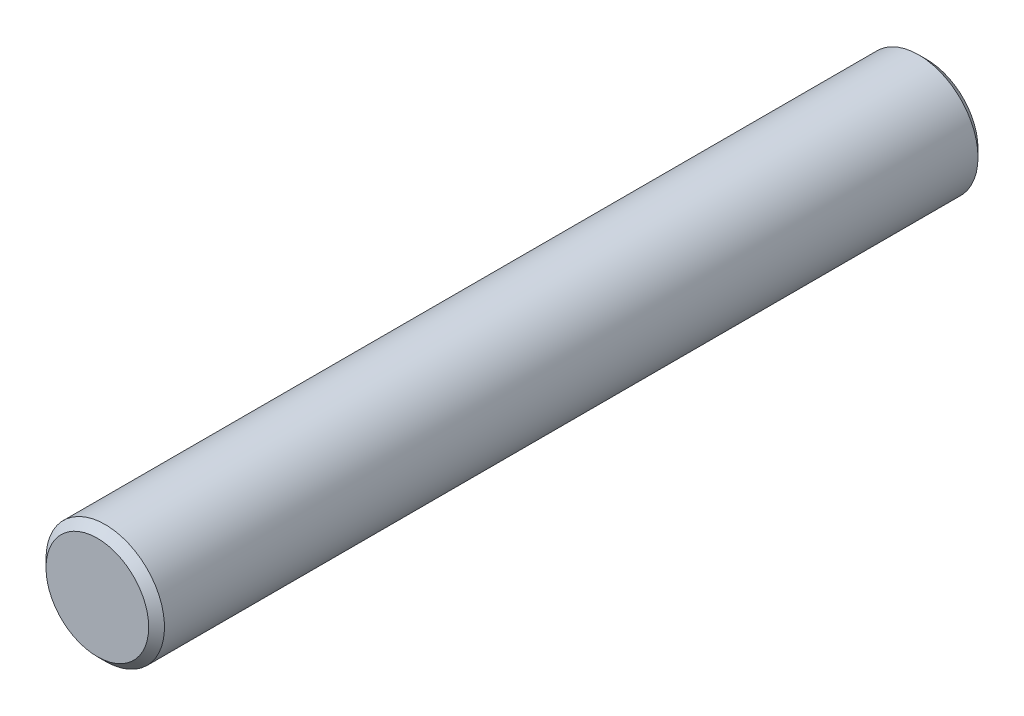
ISO-10303-21;
HEADER;
FILE_DESCRIPTION(('STEP AP214'),'2;1');
FILE_NAME('part.step','',(''),(''),'','','');
FILE_SCHEMA(('AUTOMOTIVE_DESIGN { 1 0 10303 214 1 1 1 1 }'));
ENDSEC;
DATA;
#1=APPLICATION_CONTEXT('core data for automotive mechanical design processes');
#2=APPLICATION_PROTOCOL_DEFINITION('international standard','automotive_design',2000,#1);
#3=PRODUCT_CONTEXT('',#1,'mechanical');
#4=PRODUCT('Part','Part','',(#3));
#5=PRODUCT_RELATED_PRODUCT_CATEGORY('part','',(#4));
#6=PRODUCT_DEFINITION_FORMATION('','',#4);
#7=PRODUCT_DEFINITION_CONTEXT('part definition',#1,'design');
#8=PRODUCT_DEFINITION('design','',#6,#7);
#9=PRODUCT_DEFINITION_SHAPE('','',#8);
#10=(LENGTH_UNIT() NAMED_UNIT(*) SI_UNIT(.MILLI.,.METRE.));
#11=(NAMED_UNIT(*) PLANE_ANGLE_UNIT() SI_UNIT($,.RADIAN.));
#12=(NAMED_UNIT(*) SI_UNIT($,.STERADIAN.) SOLID_ANGLE_UNIT());
#13=UNCERTAINTY_MEASURE_WITH_UNIT(LENGTH_MEASURE(1.E-05),#10,'distance_accuracy_value','');
#14=(GEOMETRIC_REPRESENTATION_CONTEXT(3) GLOBAL_UNCERTAINTY_ASSIGNED_CONTEXT((#13)) GLOBAL_UNIT_ASSIGNED_CONTEXT((#10,
#11,#12)) REPRESENTATION_CONTEXT('',''));
#15=CARTESIAN_POINT('',(0.,0.,0.));
#16=DIRECTION('',(0.,0.,1.));
#17=DIRECTION('',(1.,0.,0.));
#18=AXIS2_PLACEMENT_3D('',#15,#16,#17);
#19=CARTESIAN_POINT('',(0.,0.,10.5));
#20=DIRECTION('',(0.,0.,-1.));
#21=DIRECTION('',(-1.,0.,0.));
#22=AXIS2_PLACEMENT_3D('',#19,#20,#21);
#23=CYLINDRICAL_SURFACE('',#22,1.5);
#24=CARTESIAN_POINT('',(0.,0.,-10.3));
#25=DIRECTION('',(0.,0.,1.));
#26=DIRECTION('',(1.,0.,0.));
#27=AXIS2_PLACEMENT_3D('',#24,#25,#26);
#28=CIRCLE('',#27,1.5);
#29=CARTESIAN_POINT('',(-1.5,0.,-10.3));
#30=VERTEX_POINT('',#29);
#31=EDGE_CURVE('E51',#30,#30,#28,.T.);
#32=CARTESIAN_POINT('',(0.,0.,10.3));
#33=DIRECTION('',(0.,0.,1.));
#34=DIRECTION('',(1.,0.,0.));
#35=AXIS2_PLACEMENT_3D('',#32,#33,#34);
#36=CIRCLE('',#35,1.5);
#37=CARTESIAN_POINT('',(-1.5,0.,10.3));
#38=VERTEX_POINT('',#37);
#39=EDGE_CURVE('E54',#38,#38,#36,.F.);
#40=CARTESIAN_POINT('',(-1.5,0.,-10.3));
#41=CARTESIAN_POINT('',(-1.5,0.,-10.0854166666666));
#42=CARTESIAN_POINT('',(-1.5,0.,-9.87083333333331));
#43=CARTESIAN_POINT('',(-1.5,0.,-9.44166666666665));
#44=CARTESIAN_POINT('',(-1.5,0.,-9.22708333333332));
#45=CARTESIAN_POINT('',(-1.5,0.,-8.79791666666665));
#46=CARTESIAN_POINT('',(-1.5,0.,-8.58333333333331));
#47=CARTESIAN_POINT('',(-1.5,0.,-8.15416666666665));
#48=CARTESIAN_POINT('',(-1.5,0.,-7.93958333333331));
#49=CARTESIAN_POINT('',(-1.5,0.,-7.51041666666665));
#50=CARTESIAN_POINT('',(-1.5,0.,-7.29583333333331));
#51=CARTESIAN_POINT('',(-1.5,0.,-6.86666666666665));
#52=CARTESIAN_POINT('',(-1.5,0.,-6.65208333333332));
#53=CARTESIAN_POINT('',(-1.5,0.,-6.22291666666665));
#54=CARTESIAN_POINT('',(-1.5,0.,-6.00833333333332));
#55=CARTESIAN_POINT('',(-1.5,0.,-5.57916666666665));
#56=CARTESIAN_POINT('',(-1.5,0.,-5.36458333333332));
#57=CARTESIAN_POINT('',(-1.5,0.,-4.93541666666665));
#58=CARTESIAN_POINT('',(-1.5,0.,-4.72083333333332));
#59=CARTESIAN_POINT('',(-1.5,0.,-4.29166666666665));
#60=CARTESIAN_POINT('',(-1.5,0.,-4.07708333333332));
#61=CARTESIAN_POINT('',(-1.5,0.,-3.64791666666665));
#62=CARTESIAN_POINT('',(-1.5,0.,-3.43333333333332));
#63=CARTESIAN_POINT('',(-1.5,0.,-3.00416666666665));
#64=CARTESIAN_POINT('',(-1.5,0.,-2.78958333333332));
#65=CARTESIAN_POINT('',(-1.5,0.,-2.36041666666665));
#66=CARTESIAN_POINT('',(-1.5,0.,-2.14583333333332));
#67=CARTESIAN_POINT('',(-1.5,0.,-1.71666666666665));
#68=CARTESIAN_POINT('',(-1.5,0.,-1.50208333333332));
#69=CARTESIAN_POINT('',(-1.5,0.,-1.07291666666665));
#70=CARTESIAN_POINT('',(-1.5,0.,-0.85833333333332));
#71=CARTESIAN_POINT('',(-1.5,0.,-0.429166666666653));
#72=CARTESIAN_POINT('',(-1.5,0.,-0.21458333333332));
#73=CARTESIAN_POINT('',(-1.5,0.,0.214583333333347));
#74=CARTESIAN_POINT('',(-1.5,0.,0.429166666666681));
#75=CARTESIAN_POINT('',(-1.5,0.,0.858333333333347));
#76=CARTESIAN_POINT('',(-1.5,0.,1.07291666666668));
#77=CARTESIAN_POINT('',(-1.5,0.,1.50208333333335));
#78=CARTESIAN_POINT('',(-1.5,0.,1.71666666666668));
#79=CARTESIAN_POINT('',(-1.5,0.,2.14583333333335));
#80=CARTESIAN_POINT('',(-1.5,0.,2.36041666666668));
#81=CARTESIAN_POINT('',(-1.5,0.,2.78958333333335));
#82=CARTESIAN_POINT('',(-1.5,0.,3.00416666666668));
#83=CARTESIAN_POINT('',(-1.5,0.,3.43333333333335));
#84=CARTESIAN_POINT('',(-1.5,0.,3.64791666666668));
#85=CARTESIAN_POINT('',(-1.5,0.,4.07708333333334));
#86=CARTESIAN_POINT('',(-1.5,0.,4.29166666666668));
#87=CARTESIAN_POINT('',(-1.5,0.,4.72083333333334));
#88=CARTESIAN_POINT('',(-1.5,0.,4.93541666666668));
#89=CARTESIAN_POINT('',(-1.5,0.,5.36458333333334));
#90=CARTESIAN_POINT('',(-1.5,0.,5.57916666666668));
#91=CARTESIAN_POINT('',(-1.5,0.,6.00833333333334));
#92=CARTESIAN_POINT('',(-1.5,0.,6.22291666666668));
#93=CARTESIAN_POINT('',(-1.5,0.,6.65208333333334));
#94=CARTESIAN_POINT('',(-1.5,0.,6.86666666666668));
#95=CARTESIAN_POINT('',(-1.5,0.,7.29583333333334));
#96=CARTESIAN_POINT('',(-1.5,0.,7.51041666666667));
#97=CARTESIAN_POINT('',(-1.5,0.,7.93958333333334));
#98=CARTESIAN_POINT('',(-1.5,0.,8.15416666666668));
#99=CARTESIAN_POINT('',(-1.5,0.,8.58333333333334));
#100=CARTESIAN_POINT('',(-1.5,0.,8.79791666666668));
#101=CARTESIAN_POINT('',(-1.5,0.,9.22708333333334));
#102=CARTESIAN_POINT('',(-1.5,0.,9.44166666666668));
#103=CARTESIAN_POINT('',(-1.5,0.,9.87083333333334));
#104=CARTESIAN_POINT('',(-1.5,0.,10.0854166666667));
#105=CARTESIAN_POINT('',(-1.5,0.,10.3));
#106=B_SPLINE_CURVE_WITH_KNOTS('',3,(#40,#41,#42,#43,#44,#45,#46,#47,#48,#49,#50,#51,#52,#53,
#54,#55,#56,#57,#58,#59,#60,#61,#62,#63,#64,#65,#66,#67,#68,#69,#70,#71,#72,#73,#74,#75,#76,#77,
#78,#79,#80,#81,#82,#83,#84,#85,#86,#87,#88,#89,#90,#91,#92,#93,#94,#95,#96,#97,#98,#99,#100,
#101,#102,#103,#104,#105),.UNSPECIFIED.,.F.,.F.,(4,2,2,2,2,2,2,2,2,2,2,2,2,2,2,2,2,2,2,2,2,2,2,
2,2,2,2,2,2,2,2,2,4),(0.,0.643749999999998,1.2875,1.93125,2.575,3.21875,3.8625,4.50625,5.15,
5.79375,6.4375,7.08125,7.725,8.36875,9.01249999999999,9.65624999999999,10.3,10.94375,11.5875,
12.23125,12.875,13.51875,14.1625,14.80625,15.45,16.09375,16.7375,17.38125,18.025,18.66875,
19.3125,19.95625,20.6),.UNSPECIFIED.);
#107=EDGE_CURVE('BSEAM39',#30,#38,#106,.T.);
#108=ORIENTED_EDGE('',*,*,#31,.T.);
#109=ORIENTED_EDGE('',*,*,#39,.T.);
#110=ORIENTED_EDGE('',*,*,#107,.T.);
#111=ORIENTED_EDGE('',*,*,#107,.F.);
#112=EDGE_LOOP('',(#108,#110,#109,#111));
#113=FACE_BOUND('',#112,.T.);
#114=ADVANCED_FACE('F39',(#113),#23,.T.);
#115=CARTESIAN_POINT('',(0.,0.,10.5));
#116=DIRECTION('',(0.,0.,1.));
#117=DIRECTION('',(1.,0.,0.));
#118=AXIS2_PLACEMENT_3D('',#115,#116,#117);
#119=PLANE('',#118);
#120=CARTESIAN_POINT('',(0.,0.,10.5));
#121=DIRECTION('',(0.,0.,1.));
#122=DIRECTION('',(1.,0.,0.));
#123=AXIS2_PLACEMENT_3D('',#120,#121,#122);
#124=CIRCLE('',#123,1.30000000000001);
#125=CARTESIAN_POINT('',(1.30000000000001,0.,10.5));
#126=VERTEX_POINT('',#125);
#127=EDGE_CURVE('E10',#126,#126,#124,.T.);
#128=ORIENTED_EDGE('',*,*,#127,.T.);
#129=EDGE_LOOP('',(#128));
#130=FACE_BOUND('',#129,.T.);
#131=ADVANCED_FACE('F72',(#130),#119,.T.);
#132=CARTESIAN_POINT('',(0.,0.,-10.5));
#133=DIRECTION('',(0.,0.,1.));
#134=DIRECTION('',(1.,0.,0.));
#135=AXIS2_PLACEMENT_3D('',#132,#133,#134);
#136=PLANE('',#135);
#137=CARTESIAN_POINT('',(0.,0.,-10.5));
#138=DIRECTION('',(0.,0.,1.));
#139=DIRECTION('',(1.,0.,0.));
#140=AXIS2_PLACEMENT_3D('',#137,#138,#139);
#141=CIRCLE('',#140,1.29999999999998);
#142=CARTESIAN_POINT('',(1.29999999999998,0.,-10.5));
#143=VERTEX_POINT('',#142);
#144=EDGE_CURVE('E50',#143,#143,#141,.F.);
#145=ORIENTED_EDGE('',*,*,#144,.T.);
#146=EDGE_LOOP('',(#145));
#147=FACE_BOUND('',#146,.T.);
#148=ADVANCED_FACE('F66',(#147),#136,.F.);
#149=CARTESIAN_POINT('',(0.,0.,-10.3));
#150=DIRECTION('',(0.,0.,1.));
#151=DIRECTION('',(1.,0.,0.));
#152=AXIS2_PLACEMENT_3D('',#149,#150,#151);
#153=CONICAL_SURFACE('',#152,1.5,0.785398163397455);
#154=ORIENTED_EDGE('',*,*,#144,.F.);
#155=EDGE_LOOP('',(#154));
#156=FACE_BOUND('',#155,.T.);
#157=ORIENTED_EDGE('',*,*,#31,.F.);
#158=EDGE_LOOP('',(#157));
#159=FACE_BOUND('',#158,.T.);
#160=ADVANCED_FACE('F63',(#156,#159),#153,.T.);
#161=CARTESIAN_POINT('',(0.,0.,10.5));
#162=DIRECTION('',(0.,0.,-1.));
#163=DIRECTION('',(-1.,0.,0.));
#164=AXIS2_PLACEMENT_3D('',#161,#162,#163);
#165=CONICAL_SURFACE('',#164,1.30000000000001,0.78539816339745);
#166=ORIENTED_EDGE('',*,*,#39,.F.);
#167=EDGE_LOOP('',(#166));
#168=FACE_BOUND('',#167,.T.);
#169=ORIENTED_EDGE('',*,*,#127,.F.);
#170=EDGE_LOOP('',(#169));
#171=FACE_BOUND('',#170,.T.);
#172=ADVANCED_FACE('F45',(#168,#171),#165,.T.);
#173=CLOSED_SHELL('',(#114,#131,#148,#160,#172));
#174=MANIFOLD_SOLID_BREP('B2',#173);
#175=ADVANCED_BREP_SHAPE_REPRESENTATION('',(#18,#174),#14);
#176=SHAPE_DEFINITION_REPRESENTATION(#9,#175);
ENDSEC;
END-ISO-10303-21;
